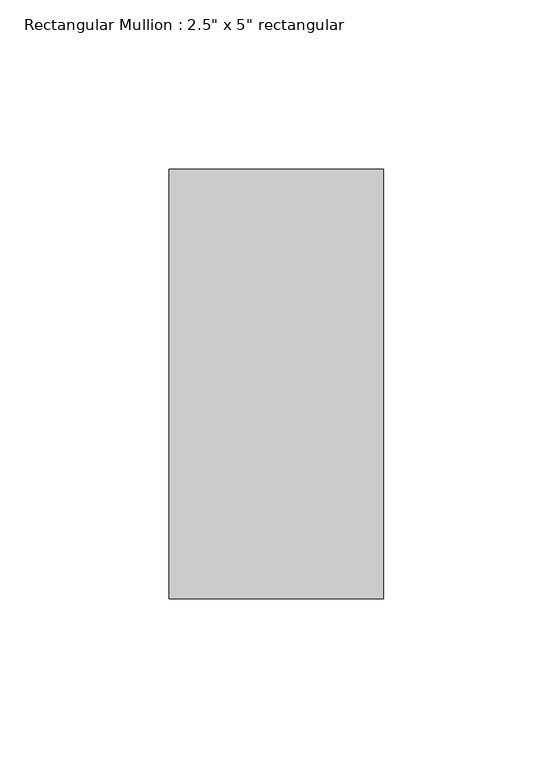
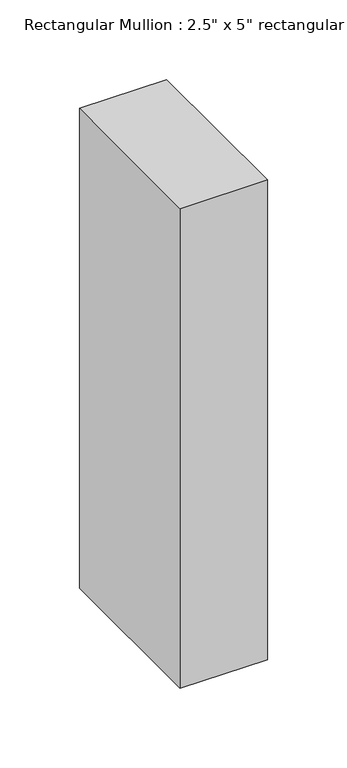
"""IFC4 building model written with IfcOpenShell, lengths in millimetres: member geometry."""

from ifc_helpers import new_model, si_unit, frame, origin, place, context, project, spatial, polyline, outline, extrude, source, transform, mapped, element, save


def member_83c59054(model_context):
    return source(origin(), model_context, "Body", "SweptSolid", [
        extrude(outline(polyline([(0.0, 63.5), (0.0, -63.5), (-63.5, -63.5), (-63.5, 63.5), (0.0, 63.5)])), frame((0.0, 0.0, -368.3), z_axis=(0.0, 0.0, 1.0), x_axis=(1.0, 0.0, 0.0)), (0.0, 0.0, 1.0), 368.3),
    ])


if __name__ == "__main__":
    model = new_model("IFC4")
    model_context = context("Model", 3, world=origin())
    ifc_project = project(units=[si_unit("LENGTHUNIT", "METRE", prefix="MILLI")], contexts=[model_context])
    site = spatial("IfcSite", under=ifc_project)
    building = spatial("IfcBuilding", under=site)
    placement = place(None, origin())
    member_shape = member_83c59054(model_context)
    element("IfcMember", 1, ObjectType="Rectangular Mullion : 2.5\" x 5\" rectangular", at=placement, inside=building, context=model_context, shape_type="MappedRepresentation", body=[
        mapped(member_shape, transform((0.0, 0.0, 0.0), x_axis=(1.0, 0.0, 0.0), y_axis=(0.0, 1.0, 0.0), z_axis=(0.0, 0.0, 1.0))),
    ])
    save(model, "model.ifc")

# Revit data of these elements
# Type "Rectangular Mullion : 2.5\" x 5\" rectangular"
#   built-in parameter 1007304 = 0.416667 (stored number, unit not read)
#   built-in parameter 1007301 = 0.104167 (stored number, unit not read)
#   built-in parameter 1007300 = 0.104167 (stored number, unit not read)
# Element 1 (IfcMember, "Rectangular Mullion : 2.5\" x 5\" rectangular")
#   Materials on its faces: "Aluminum"
# Materials
#   "Aluminum": class "Metal", colour RGB 247 247 247, transparency 0, Description = "Aluminum 6061", Cost = 0
